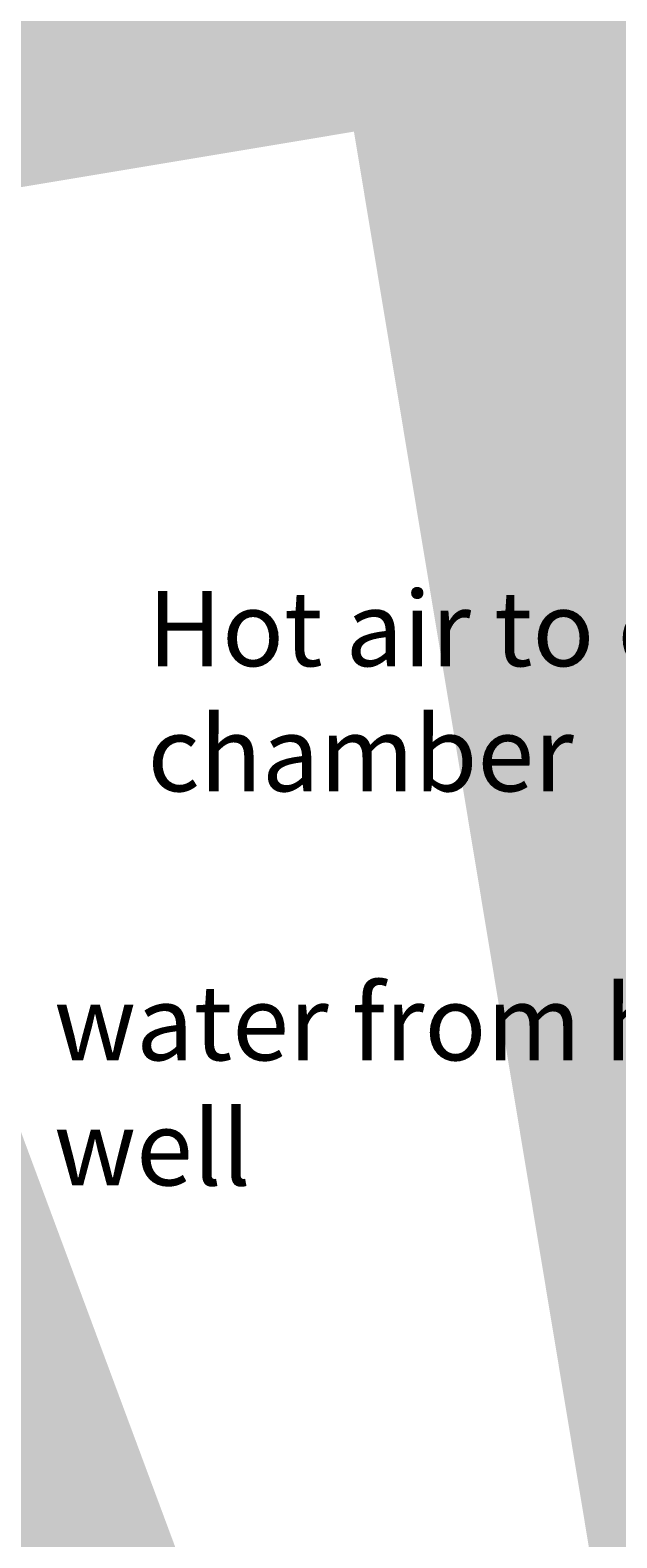
# Model space of a CAD drawing. Units: millimetres. Extents: x -22994 to 29398, y -19990 to 20176.
# Tile 22 of 135: x 5 to 37, y 99 to 180. Entities that reach past the tile are written whole.
import ezdxf

# ---------------------------------------------------------------- set-up
doc = ezdxf.new("R2010")
doc.units = ezdxf.units.MM
doc.header["$MEASUREMENT"] = 0
doc.layers.add('M-ANNO-TEXT', color=7, linetype='Continuous', lineweight=25)
doc.layers.add('M-DIMS', color=2, linetype='Continuous', lineweight=18)
doc.styles.get("Standard").update_dxf_attribs({"font": 'arial.ttf'})
doc.dimstyles.get("Standard").update_dxf_attribs({"dimtxt": 0.18, "dimasz": 10000, "dimexe": 0.18, "dimexo": 0.0625, "dimgap": 0.09, "dimtad": 0, "dimtih": 1, "dimtoh": 1, "dimdec": 0, "dimzin": 0, "dimdsep": 46, "dimtxsty": 'Standard', "dimcen": 0.09, "dimadec": 0, "dimazin": 0, "dimtfac": 1, "dimtdec": 0, "dimtofl": 0, "dimtmove": 0, "dimatfit": 3, "dimfxl": 1, "dimtolj": 1, "dimtzin": 0, "dimlwd": 30, "dimarcsym": 0})

# ---------------------------------------------------------------- blocks, each defined once
blk = doc.blocks.new('*D2')
at = {"layer": 'Defpoints', "color": 0, "transparency": 16777216}
for p in [(6.677, 10.271), (290.852, 10.271), (290.852, -5.079)]:
    blk.add_point(p, dxfattribs=at)
at = {"layer": 'M-DIMS', "color": 0, "lineweight": -2, "transparency": 16777216}
for p, q in [((6.677, 10.209), (6.677, -5.259)), ((290.852, 10.209), (290.852, -5.259))]:
    blk.add_line(p, q, dxfattribs=at)
at = {"layer": 'M-DIMS', "color": 0, "lineweight": 30, "transparency": 16777216}
for p, q in [((-9993.323, -5.079), (-19993.323, -5.079)), ((10290.852, -5.079), (20290.852, -5.079))]:
    blk.add_line(p, q, dxfattribs=at)
at = {"layer": 'M-DIMS', "color": 0, "transparency": 16777216}
for points in [[(-9993.323, 1661.588), (-9993.323, -1671.745), (6.677, -5.079)], [(10290.852, 1661.588), (10290.852, -1671.745), (290.852, -5.079)]]:
    blk.add_solid(points, dxfattribs=at)
at = {"layer": 'M-DIMS', "color": 0, "transparency": 16777216, "insert": (148.765, -5.079), "char_height": 0.18, "attachment_point": 5}
blk.add_mtext('\\A1;284.2', dxfattribs=at)
blk = doc.blocks.new('*D3')
at = {"layer": 'Defpoints', "color": 0, "transparency": 16777216}
for p in [(110.265, 204.165), (110.265, 176.366), (95.833, 127.967)]:
    blk.add_point(p, dxfattribs=at)
at = {"layer": 'M-DIMS', "color": 0, "lineweight": 30, "transparency": 16777216}
for p, q in [((-9904.167, 204.165), (-19904.167, 204.165)), ((10110.265, 204.165), (20110.265, 204.165))]:
    blk.add_line(p, q, dxfattribs=at)
at = {"layer": 'M-DIMS', "color": 0, "lineweight": -2, "transparency": 16777216}
for p, q in [((95.833, 128.03), (95.833, 204.345)), ((110.265, 176.429), (110.265, 204.345))]:
    blk.add_line(p, q, dxfattribs=at)
at = {"layer": 'M-DIMS', "color": 0, "transparency": 16777216}
for points in [[(-9904.167, 1870.832), (-9904.167, -1462.501), (95.833, 204.165)], [(10110.265, 1870.832), (10110.265, -1462.501), (110.265, 204.165)]]:
    blk.add_solid(points, dxfattribs=at)
at = {"layer": 'M-DIMS', "color": 0, "transparency": 16777216, "insert": (103.049, 204.165), "char_height": 0.18, "attachment_point": 5}
blk.add_mtext('\\A1;14.432', dxfattribs=at)
blk = doc.blocks.new('*D4')
at = {"layer": 'Defpoints', "color": 0, "transparency": 16777216}
for p in [(116.265, 204.165), (110.265, 176.366), (116.265, 176.366)]:
    blk.add_point(p, dxfattribs=at)
at = {"layer": 'M-DIMS', "color": 0, "lineweight": 30, "transparency": 16777216}
for p, q in [((-9889.735, 204.165), (-19889.735, 204.165)), ((10116.265, 204.165), (20116.265, 204.165))]:
    blk.add_line(p, q, dxfattribs=at)
at = {"layer": 'M-DIMS', "color": 0, "lineweight": -2, "transparency": 16777216}
for p, q in [((110.265, 176.429), (110.265, 204.345)), ((116.265, 176.429), (116.265, 204.345))]:
    blk.add_line(p, q, dxfattribs=at)
at = {"layer": 'M-DIMS', "color": 0, "transparency": 16777216}
for points in [[(-9889.735, 1870.832), (-9889.735, -1462.501), (110.265, 204.165)], [(10116.265, 1870.832), (10116.265, -1462.501), (116.265, 204.165)]]:
    blk.add_solid(points, dxfattribs=at)
at = {"layer": 'M-DIMS', "color": 0, "transparency": 16777216, "insert": (113.265, 204.165), "char_height": 0.18, "attachment_point": 5}
blk.add_mtext('\\A1;6', dxfattribs=at)
blk = doc.blocks.new('*D5')
at = {"layer": 'Defpoints', "color": 0, "transparency": 16777216}
for p in [(181.265, 204.165), (116.265, 176.366), (181.265, 176.366)]:
    blk.add_point(p, dxfattribs=at)
at = {"layer": 'M-DIMS', "color": 0, "lineweight": 30, "transparency": 16777216}
for p, q in [((-9883.735, 204.165), (-19883.735, 204.165)), ((10181.265, 204.165), (20181.265, 204.165))]:
    blk.add_line(p, q, dxfattribs=at)
at = {"layer": 'M-DIMS', "color": 0, "lineweight": -2, "transparency": 16777216}
for p, q in [((116.265, 176.429), (116.265, 204.345)), ((181.265, 176.429), (181.265, 204.345))]:
    blk.add_line(p, q, dxfattribs=at)
at = {"layer": 'M-DIMS', "color": 0, "transparency": 16777216}
for points in [[(-9883.735, 1870.832), (-9883.735, -1462.501), (116.265, 204.165)], [(10181.265, 1870.832), (10181.265, -1462.501), (181.265, 204.165)]]:
    blk.add_solid(points, dxfattribs=at)
at = {"layer": 'M-DIMS', "color": 0, "transparency": 16777216, "insert": (148.765, 204.165), "char_height": 0.18, "attachment_point": 5}
blk.add_mtext('\\A1;65', dxfattribs=at)
blk = doc.blocks.new('*D6')
at = {"layer": 'Defpoints', "color": 0, "transparency": 16777216}
for p in [(187.265, 204.165), (181.265, 176.366), (187.265, 176.366)]:
    blk.add_point(p, dxfattribs=at)
at = {"layer": 'M-DIMS', "color": 0, "lineweight": 30, "transparency": 16777216}
for p, q in [((-9818.735, 204.165), (-19818.735, 204.165)), ((10187.265, 204.165), (20187.265, 204.165))]:
    blk.add_line(p, q, dxfattribs=at)
at = {"layer": 'M-DIMS', "color": 0, "lineweight": -2, "transparency": 16777216}
for p, q in [((181.265, 176.429), (181.265, 204.345)), ((187.265, 176.429), (187.265, 204.345))]:
    blk.add_line(p, q, dxfattribs=at)
at = {"layer": 'M-DIMS', "color": 0, "transparency": 16777216}
for points in [[(-9818.735, 1870.832), (-9818.735, -1462.501), (181.265, 204.165)], [(10187.265, 1870.832), (10187.265, -1462.501), (187.265, 204.165)]]:
    blk.add_solid(points, dxfattribs=at)
at = {"layer": 'M-DIMS', "color": 0, "transparency": 16777216, "insert": (184.265, 204.165), "char_height": 0.18, "attachment_point": 5}
blk.add_mtext('\\A1;6', dxfattribs=at)
blk = doc.blocks.new('*D7')
at = {"layer": 'Defpoints', "color": 0, "transparency": 16777216}
for p in [(201.697, 204.165), (187.265, 176.366), (201.697, 127.967)]:
    blk.add_point(p, dxfattribs=at)
at = {"layer": 'M-DIMS', "color": 0, "lineweight": 30, "transparency": 16777216}
for p, q in [((-9812.735, 204.165), (-19812.735, 204.165)), ((10201.697, 204.165), (20201.697, 204.165))]:
    blk.add_line(p, q, dxfattribs=at)
at = {"layer": 'M-DIMS', "color": 0, "lineweight": -2, "transparency": 16777216}
for p, q in [((187.265, 176.429), (187.265, 204.345)), ((201.697, 128.03), (201.697, 204.345))]:
    blk.add_line(p, q, dxfattribs=at)
at = {"layer": 'M-DIMS', "color": 0, "transparency": 16777216}
for points in [[(-9812.735, 1870.832), (-9812.735, -1462.501), (187.265, 204.165)], [(10201.697, 1870.832), (10201.697, -1462.501), (201.697, 204.165)]]:
    blk.add_solid(points, dxfattribs=at)
at = {"layer": 'M-DIMS', "color": 0, "transparency": 16777216, "insert": (194.481, 204.165), "char_height": 0.18, "attachment_point": 5}
blk.add_mtext('\\A1;14.432', dxfattribs=at)
blk = doc.blocks.new('*D8')
at = {"layer": 'Defpoints', "color": 0, "transparency": 16777216}
for p in [(227.648, 204.165), (227.648, 146.73), (201.697, 127.967)]:
    blk.add_point(p, dxfattribs=at)
at = {"layer": 'M-DIMS', "color": 0, "lineweight": 30, "transparency": 16777216}
for p, q in [((-9798.303, 204.165), (-19798.303, 204.165)), ((10227.648, 204.165), (20227.648, 204.165))]:
    blk.add_line(p, q, dxfattribs=at)
at = {"layer": 'M-DIMS', "color": 0, "lineweight": -2, "transparency": 16777216}
for p, q in [((201.697, 128.03), (201.697, 204.345)), ((227.648, 146.792), (227.648, 204.345))]:
    blk.add_line(p, q, dxfattribs=at)
at = {"layer": 'M-DIMS', "color": 0, "transparency": 16777216}
for points in [[(-9798.303, 1870.832), (-9798.303, -1462.501), (201.697, 204.165)], [(10227.648, 1870.832), (10227.648, -1462.501), (227.648, 204.165)]]:
    blk.add_solid(points, dxfattribs=at)
at = {"layer": 'M-DIMS', "color": 0, "transparency": 16777216, "insert": (214.673, 204.165), "char_height": 0.18, "attachment_point": 5}
blk.add_mtext('\\A1;25.95', dxfattribs=at)
blk = doc.blocks.new('*D9')
at = {"layer": 'Defpoints', "color": 0, "transparency": 16777216}
for p in [(187.265, 176.366), (306.202, 176.366), (290.852, 10.271)]:
    blk.add_point(p, dxfattribs=at)
at = {"layer": 'M-DIMS', "color": 0, "lineweight": 30, "transparency": 16777216}
for p, q in [((306.202, 10176.366), (306.202, 20176.366)), ((306.202, -9989.729), (306.202, -19989.729))]:
    blk.add_line(p, q, dxfattribs=at)
at = {"layer": 'M-DIMS', "color": 0, "lineweight": -2, "transparency": 16777216}
for p, q in [((187.327, 176.366), (306.382, 176.366)), ((290.915, 10.271), (306.382, 10.271))]:
    blk.add_line(p, q, dxfattribs=at)
at = {"layer": 'M-DIMS', "color": 0, "transparency": 16777216}
for points in [[(-1360.465, 10176.366), (1972.869, 10176.366), (306.202, 176.366)], [(-1360.465, -9989.729), (1972.869, -9989.729), (306.202, 10.271)]]:
    blk.add_solid(points, dxfattribs=at)
at = {"layer": 'M-DIMS', "color": 0, "transparency": 16777216, "insert": (306.202, 93.319), "char_height": 0.18, "attachment_point": 5}
blk.add_mtext('\\A1;166.1', dxfattribs=at)
blk = doc.blocks.new('*D10')
at = {"layer": 'Defpoints', "color": 0, "transparency": 16777216}
for p in [(125.65, 136.071), (133.346, 136.071), (133.346, -5.079)]:
    blk.add_point(p, dxfattribs=at)
at = {"layer": 'M-DIMS', "color": 0, "lineweight": -2, "transparency": 16777216}
for p, q in [((125.65, 136.009), (125.65, -5.259)), ((133.346, 136.009), (133.346, -5.259))]:
    blk.add_line(p, q, dxfattribs=at)
at = {"layer": 'M-DIMS', "color": 0, "lineweight": 30, "transparency": 16777216}
for p, q in [((-9874.35, -5.079), (-19874.35, -5.079)), ((10133.346, -5.079), (20133.346, -5.079))]:
    blk.add_line(p, q, dxfattribs=at)
at = {"layer": 'M-DIMS', "color": 0, "transparency": 16777216}
for points in [[(-9874.35, 1661.588), (-9874.35, -1671.745), (125.65, -5.079)], [(10133.346, 1661.588), (10133.346, -1671.745), (133.346, -5.079)]]:
    blk.add_solid(points, dxfattribs=at)
at = {"layer": 'M-DIMS', "color": 0, "transparency": 16777216, "insert": (129.498, -5.079), "char_height": 0.18, "attachment_point": 5}
blk.add_mtext('\\A1;7.696', dxfattribs=at)
blk = doc.blocks.new('*D11')
at = {"layer": 'Defpoints', "color": 0, "transparency": 16777216}
for p in [(133.346, 136.071), (135.65, 136.071), (135.65, -5.079)]:
    blk.add_point(p, dxfattribs=at)
at = {"layer": 'M-DIMS', "color": 0, "lineweight": -2, "transparency": 16777216}
for p, q in [((133.346, 136.009), (133.346, -5.259)), ((135.65, 136.009), (135.65, -5.259))]:
    blk.add_line(p, q, dxfattribs=at)
at = {"layer": 'M-DIMS', "color": 0, "lineweight": 30, "transparency": 16777216}
for p, q in [((-9866.654, -5.079), (-19866.654, -5.079)), ((10135.65, -5.079), (20135.65, -5.079))]:
    blk.add_line(p, q, dxfattribs=at)
at = {"layer": 'M-DIMS', "color": 0, "transparency": 16777216}
for points in [[(-9866.654, 1661.588), (-9866.654, -1671.745), (133.346, -5.079)], [(10135.65, 1661.588), (10135.65, -1671.745), (135.65, -5.079)]]:
    blk.add_solid(points, dxfattribs=at)
at = {"layer": 'M-DIMS', "color": 0, "transparency": 16777216, "insert": (134.498, -5.079), "char_height": 0.18, "attachment_point": 5}
blk.add_mtext('\\A1;2.304', dxfattribs=at)
blk = doc.blocks.new('*D12')
at = {"layer": 'Defpoints', "color": 0, "transparency": 16777216}
for p in [(135.65, 136.071), (145.65, 136.071), (145.65, -5.079)]:
    blk.add_point(p, dxfattribs=at)
at = {"layer": 'M-DIMS', "color": 0, "lineweight": -2, "transparency": 16777216}
for p, q in [((135.65, 136.009), (135.65, -5.259)), ((145.65, 136.009), (145.65, -5.259))]:
    blk.add_line(p, q, dxfattribs=at)
at = {"layer": 'M-DIMS', "color": 0, "lineweight": 30, "transparency": 16777216}
for p, q in [((-9864.35, -5.079), (-19864.35, -5.079)), ((10145.65, -5.079), (20145.65, -5.079))]:
    blk.add_line(p, q, dxfattribs=at)
at = {"layer": 'M-DIMS', "color": 0, "transparency": 16777216}
for points in [[(-9864.35, 1661.588), (-9864.35, -1671.745), (135.65, -5.079)], [(10145.65, 1661.588), (10145.65, -1671.745), (145.65, -5.079)]]:
    blk.add_solid(points, dxfattribs=at)
at = {"layer": 'M-DIMS', "color": 0, "transparency": 16777216, "insert": (140.65, -5.079), "char_height": 0.18, "attachment_point": 5}
blk.add_mtext('\\A1;10', dxfattribs=at)
blk = doc.blocks.new('*D13')
at = {"layer": 'Defpoints', "color": 0, "transparency": 16777216}
for p in [(145.65, 136.071), (155.65, 136.071), (155.65, -5.079)]:
    blk.add_point(p, dxfattribs=at)
at = {"layer": 'M-DIMS', "color": 0, "lineweight": -2, "transparency": 16777216}
for p, q in [((145.65, 136.009), (145.65, -5.259)), ((155.65, 136.009), (155.65, -5.259))]:
    blk.add_line(p, q, dxfattribs=at)
at = {"layer": 'M-DIMS', "color": 0, "lineweight": 30, "transparency": 16777216}
for p, q in [((-9854.35, -5.079), (-19854.35, -5.079)), ((10155.65, -5.079), (20155.65, -5.079))]:
    blk.add_line(p, q, dxfattribs=at)
at = {"layer": 'M-DIMS', "color": 0, "transparency": 16777216}
for points in [[(-9854.35, 1661.588), (-9854.35, -1671.745), (145.65, -5.079)], [(10155.65, 1661.588), (10155.65, -1671.745), (155.65, -5.079)]]:
    blk.add_solid(points, dxfattribs=at)
at = {"layer": 'M-DIMS', "color": 0, "transparency": 16777216, "insert": (150.65, -5.079), "char_height": 0.18, "attachment_point": 5}
blk.add_mtext('\\A1;10', dxfattribs=at)
blk = doc.blocks.new('*D14')
at = {"layer": 'Defpoints', "color": 0, "transparency": 16777216}
for p in [(155.65, 136.071), (165.65, 136.071), (165.65, -5.079)]:
    blk.add_point(p, dxfattribs=at)
at = {"layer": 'M-DIMS', "color": 0, "lineweight": -2, "transparency": 16777216}
for p, q in [((155.65, 136.009), (155.65, -5.259)), ((165.65, 136.009), (165.65, -5.259))]:
    blk.add_line(p, q, dxfattribs=at)
at = {"layer": 'M-DIMS', "color": 0, "lineweight": 30, "transparency": 16777216}
for p, q in [((-9844.35, -5.079), (-19844.35, -5.079)), ((10165.65, -5.079), (20165.65, -5.079))]:
    blk.add_line(p, q, dxfattribs=at)
at = {"layer": 'M-DIMS', "color": 0, "transparency": 16777216}
for points in [[(-9844.35, 1661.588), (-9844.35, -1671.745), (155.65, -5.079)], [(10165.65, 1661.588), (10165.65, -1671.745), (165.65, -5.079)]]:
    blk.add_solid(points, dxfattribs=at)
at = {"layer": 'M-DIMS', "color": 0, "transparency": 16777216, "insert": (160.65, -5.079), "char_height": 0.18, "attachment_point": 5}
blk.add_mtext('\\A1;10', dxfattribs=at)
blk = doc.blocks.new('*D15')
at = {"layer": 'Defpoints', "color": 0, "transparency": 16777216}
for p in [(173.346, 154.788), (173.346, 136.071), (306.202, 136.071)]:
    blk.add_point(p, dxfattribs=at)
at = {"layer": 'M-DIMS', "color": 0, "lineweight": 30, "transparency": 16777216}
for p, q in [((306.202, 10154.788), (306.202, 20154.788)), ((306.202, -9863.929), (306.202, -19863.929))]:
    blk.add_line(p, q, dxfattribs=at)
at = {"layer": 'M-DIMS', "color": 0, "lineweight": -2, "transparency": 16777216}
for p, q in [((173.408, 154.788), (306.382, 154.788)), ((173.408, 136.071), (306.382, 136.071))]:
    blk.add_line(p, q, dxfattribs=at)
at = {"layer": 'M-DIMS', "color": 0, "transparency": 16777216}
for points in [[(-1360.465, 10154.788), (1972.869, 10154.788), (306.202, 154.788)], [(-1360.465, -9863.929), (1972.869, -9863.929), (306.202, 136.071)]]:
    blk.add_solid(points, dxfattribs=at)
at = {"layer": 'M-DIMS', "color": 0, "transparency": 16777216, "insert": (306.202, 145.43), "char_height": 0.18, "attachment_point": 5}
blk.add_mtext('\\A1;18.717', dxfattribs=at)
blk = doc.blocks.new('*D16')
at = {"layer": 'Defpoints', "color": 0, "transparency": 16777216}
for p in [(120.17, 204.165), (110.466, 48.035), (120.17, 48.035)]:
    blk.add_point(p, dxfattribs=at)
at = {"layer": 'M-DIMS', "color": 0, "lineweight": 30, "transparency": 16777216}
for p, q in [((-9889.534, 204.165), (-19889.534, 204.165)), ((10120.17, 204.165), (20120.17, 204.165))]:
    blk.add_line(p, q, dxfattribs=at)
at = {"layer": 'M-DIMS', "color": 0, "lineweight": -2, "transparency": 16777216}
for p, q in [((110.466, 48.097), (110.466, 204.345)), ((120.17, 48.097), (120.17, 204.345))]:
    blk.add_line(p, q, dxfattribs=at)
at = {"layer": 'M-DIMS', "color": 0, "transparency": 16777216}
for points in [[(-9889.534, 1870.832), (-9889.534, -1462.501), (110.466, 204.165)], [(10120.17, 1870.832), (10120.17, -1462.501), (120.17, 204.165)]]:
    blk.add_solid(points, dxfattribs=at)
at = {"layer": 'M-DIMS', "color": 0, "transparency": 16777216, "insert": (115.318, 204.165), "char_height": 0.18, "attachment_point": 5}
blk.add_mtext('\\A1;9.704', dxfattribs=at)
blk = doc.blocks.new('*D17')
at = {"layer": 'Defpoints', "color": 0, "transparency": 16777216}
for p in [(126.17, 204.165), (120.17, 48.035), (126.17, 48.035)]:
    blk.add_point(p, dxfattribs=at)
at = {"layer": 'M-DIMS', "color": 0, "lineweight": 30, "transparency": 16777216}
for p, q in [((-9879.83, 204.165), (-19879.83, 204.165)), ((10126.17, 204.165), (20126.17, 204.165))]:
    blk.add_line(p, q, dxfattribs=at)
at = {"layer": 'M-DIMS', "color": 0, "lineweight": -2, "transparency": 16777216}
for p, q in [((120.17, 48.097), (120.17, 204.345)), ((126.17, 48.097), (126.17, 204.345))]:
    blk.add_line(p, q, dxfattribs=at)
at = {"layer": 'M-DIMS', "color": 0, "transparency": 16777216}
for points in [[(-9879.83, 1870.832), (-9879.83, -1462.501), (120.17, 204.165)], [(10126.17, 1870.832), (10126.17, -1462.501), (126.17, 204.165)]]:
    blk.add_solid(points, dxfattribs=at)
at = {"layer": 'M-DIMS', "color": 0, "transparency": 16777216, "insert": (123.17, 204.165), "char_height": 0.18, "attachment_point": 5}
blk.add_mtext('\\A1;6', dxfattribs=at)
blk = doc.blocks.new('*D18')
at = {"layer": 'Defpoints', "color": 0, "transparency": 16777216}
for p in [(132.17, 204.165), (126.17, 48.035), (132.17, 48.035)]:
    blk.add_point(p, dxfattribs=at)
at = {"layer": 'M-DIMS', "color": 0, "lineweight": 30, "transparency": 16777216}
for p, q in [((-9873.83, 204.165), (-19873.83, 204.165)), ((10132.17, 204.165), (20132.17, 204.165))]:
    blk.add_line(p, q, dxfattribs=at)
at = {"layer": 'M-DIMS', "color": 0, "lineweight": -2, "transparency": 16777216}
for p, q in [((126.17, 48.097), (126.17, 204.345)), ((132.17, 48.097), (132.17, 204.345))]:
    blk.add_line(p, q, dxfattribs=at)
at = {"layer": 'M-DIMS', "color": 0, "transparency": 16777216}
for points in [[(-9873.83, 1870.832), (-9873.83, -1462.501), (126.17, 204.165)], [(10132.17, 1870.832), (10132.17, -1462.501), (132.17, 204.165)]]:
    blk.add_solid(points, dxfattribs=at)
at = {"layer": 'M-DIMS', "color": 0, "transparency": 16777216, "insert": (129.17, 204.165), "char_height": 0.18, "attachment_point": 5}
blk.add_mtext('\\A1;6', dxfattribs=at)
blk = doc.blocks.new('*D19')
at = {"layer": 'Defpoints', "color": 0, "transparency": 16777216}
for p in [(138.17, 204.165), (132.17, 48.035), (138.17, 48.035)]:
    blk.add_point(p, dxfattribs=at)
at = {"layer": 'M-DIMS', "color": 0, "lineweight": 30, "transparency": 16777216}
for p, q in [((-9867.83, 204.165), (-19867.83, 204.165)), ((10138.17, 204.165), (20138.17, 204.165))]:
    blk.add_line(p, q, dxfattribs=at)
at = {"layer": 'M-DIMS', "color": 0, "lineweight": -2, "transparency": 16777216}
for p, q in [((132.17, 48.097), (132.17, 204.345)), ((138.17, 48.097), (138.17, 204.345))]:
    blk.add_line(p, q, dxfattribs=at)
at = {"layer": 'M-DIMS', "color": 0, "transparency": 16777216}
for points in [[(-9867.83, 1870.832), (-9867.83, -1462.501), (132.17, 204.165)], [(10138.17, 1870.832), (10138.17, -1462.501), (138.17, 204.165)]]:
    blk.add_solid(points, dxfattribs=at)
at = {"layer": 'M-DIMS', "color": 0, "transparency": 16777216, "insert": (135.17, 204.165), "char_height": 0.18, "attachment_point": 5}
blk.add_mtext('\\A1;6', dxfattribs=at)
blk = doc.blocks.new('*D20')
at = {"layer": 'Defpoints', "color": 0, "transparency": 16777216}
for p in [(144.17, 204.165), (138.17, 48.035), (144.17, 48.035)]:
    blk.add_point(p, dxfattribs=at)
at = {"layer": 'M-DIMS', "color": 0, "lineweight": 30, "transparency": 16777216}
for p, q in [((-9861.83, 204.165), (-19861.83, 204.165)), ((10144.17, 204.165), (20144.17, 204.165))]:
    blk.add_line(p, q, dxfattribs=at)
at = {"layer": 'M-DIMS', "color": 0, "lineweight": -2, "transparency": 16777216}
for p, q in [((138.17, 48.097), (138.17, 204.345)), ((144.17, 48.097), (144.17, 204.345))]:
    blk.add_line(p, q, dxfattribs=at)
at = {"layer": 'M-DIMS', "color": 0, "transparency": 16777216}
for points in [[(-9861.83, 1870.832), (-9861.83, -1462.501), (138.17, 204.165)], [(10144.17, 1870.832), (10144.17, -1462.501), (144.17, 204.165)]]:
    blk.add_solid(points, dxfattribs=at)
at = {"layer": 'M-DIMS', "color": 0, "transparency": 16777216, "insert": (141.17, 204.165), "char_height": 0.18, "attachment_point": 5}
blk.add_mtext('\\A1;6', dxfattribs=at)
blk = doc.blocks.new('*D21')
at = {"layer": 'Defpoints', "color": 0, "transparency": 16777216}
for p in [(149.116, 204.165), (144.17, 48.035), (149.116, 48.035)]:
    blk.add_point(p, dxfattribs=at)
at = {"layer": 'M-DIMS', "color": 0, "lineweight": 30, "transparency": 16777216}
for p, q in [((-9855.83, 204.165), (-19855.83, 204.165)), ((10149.116, 204.165), (20149.116, 204.165))]:
    blk.add_line(p, q, dxfattribs=at)
at = {"layer": 'M-DIMS', "color": 0, "lineweight": -2, "transparency": 16777216}
for p, q in [((144.17, 48.097), (144.17, 204.345)), ((149.116, 48.097), (149.116, 204.345))]:
    blk.add_line(p, q, dxfattribs=at)
at = {"layer": 'M-DIMS', "color": 0, "transparency": 16777216}
for points in [[(-9855.83, 1870.832), (-9855.83, -1462.501), (144.17, 204.165)], [(10149.116, 1870.832), (10149.116, -1462.501), (149.116, 204.165)]]:
    blk.add_solid(points, dxfattribs=at)
at = {"layer": 'M-DIMS', "color": 0, "transparency": 16777216, "insert": (146.643, 204.165), "char_height": 0.18, "attachment_point": 5}
blk.add_mtext('\\A1;4.945', dxfattribs=at)
blk = doc.blocks.new('*D22')
at = {"layer": 'Defpoints', "color": 0, "transparency": 16777216}
for p in [(149.116, 30.99), (155.116, 30.99), (155.116, -5.079)]:
    blk.add_point(p, dxfattribs=at)
at = {"layer": 'M-DIMS', "color": 0, "lineweight": -2, "transparency": 16777216}
for p, q in [((149.116, 30.927), (149.116, -5.259)), ((155.116, 30.927), (155.116, -5.259))]:
    blk.add_line(p, q, dxfattribs=at)
at = {"layer": 'M-DIMS', "color": 0, "lineweight": 30, "transparency": 16777216}
for p, q in [((-9850.884, -5.079), (-19850.884, -5.079)), ((10155.116, -5.079), (20155.116, -5.079))]:
    blk.add_line(p, q, dxfattribs=at)
at = {"layer": 'M-DIMS', "color": 0, "transparency": 16777216}
for points in [[(-9850.884, 1661.588), (-9850.884, -1671.745), (149.116, -5.079)], [(10155.116, 1661.588), (10155.116, -1671.745), (155.116, -5.079)]]:
    blk.add_solid(points, dxfattribs=at)
at = {"layer": 'M-DIMS', "color": 0, "transparency": 16777216, "insert": (152.116, -5.079), "char_height": 0.18, "attachment_point": 5}
blk.add_mtext('\\A1;6', dxfattribs=at)
blk = doc.blocks.new('*D23')
at = {"layer": 'Defpoints', "color": 0, "transparency": 16777216}
for p in [(155.116, 30.99), (161.116, 30.99), (161.116, -5.079)]:
    blk.add_point(p, dxfattribs=at)
at = {"layer": 'M-DIMS', "color": 0, "lineweight": -2, "transparency": 16777216}
for p, q in [((155.116, 30.927), (155.116, -5.259)), ((161.116, 30.927), (161.116, -5.259))]:
    blk.add_line(p, q, dxfattribs=at)
at = {"layer": 'M-DIMS', "color": 0, "lineweight": 30, "transparency": 16777216}
for p, q in [((-9844.884, -5.079), (-19844.884, -5.079)), ((10161.116, -5.079), (20161.116, -5.079))]:
    blk.add_line(p, q, dxfattribs=at)
at = {"layer": 'M-DIMS', "color": 0, "transparency": 16777216}
for points in [[(-9844.884, 1661.588), (-9844.884, -1671.745), (155.116, -5.079)], [(10161.116, 1661.588), (10161.116, -1671.745), (161.116, -5.079)]]:
    blk.add_solid(points, dxfattribs=at)
at = {"layer": 'M-DIMS', "color": 0, "transparency": 16777216, "insert": (158.116, -5.079), "char_height": 0.18, "attachment_point": 5}
blk.add_mtext('\\A1;6', dxfattribs=at)
blk = doc.blocks.new('*D24')
at = {"layer": 'Defpoints', "color": 0, "transparency": 16777216}
for p in [(161.116, 30.99), (166.439, 30.99), (166.439, -5.079)]:
    blk.add_point(p, dxfattribs=at)
at = {"layer": 'M-DIMS', "color": 0, "lineweight": -2, "transparency": 16777216}
for p, q in [((161.116, 30.927), (161.116, -5.259)), ((166.439, 30.927), (166.439, -5.259))]:
    blk.add_line(p, q, dxfattribs=at)
at = {"layer": 'M-DIMS', "color": 0, "lineweight": 30, "transparency": 16777216}
for p, q in [((-9838.884, -5.079), (-19838.884, -5.079)), ((10166.439, -5.079), (20166.439, -5.079))]:
    blk.add_line(p, q, dxfattribs=at)
at = {"layer": 'M-DIMS', "color": 0, "transparency": 16777216}
for points in [[(-9838.884, 1661.588), (-9838.884, -1671.745), (161.116, -5.079)], [(10166.439, 1661.588), (10166.439, -1671.745), (166.439, -5.079)]]:
    blk.add_solid(points, dxfattribs=at)
at = {"layer": 'M-DIMS', "color": 0, "transparency": 16777216, "insert": (163.777, -5.079), "char_height": 0.18, "attachment_point": 5}
blk.add_mtext('\\A1;5.323', dxfattribs=at)
blk = doc.blocks.new('*D25')
at = {"layer": 'Defpoints', "color": 0, "transparency": 16777216}
for p in [(166.439, 30.99), (172.439, 30.99), (172.439, -5.079)]:
    blk.add_point(p, dxfattribs=at)
at = {"layer": 'M-DIMS', "color": 0, "lineweight": -2, "transparency": 16777216}
for p, q in [((166.439, 30.927), (166.439, -5.259)), ((172.439, 30.927), (172.439, -5.259))]:
    blk.add_line(p, q, dxfattribs=at)
at = {"layer": 'M-DIMS', "color": 0, "lineweight": 30, "transparency": 16777216}
for p, q in [((-9833.561, -5.079), (-19833.561, -5.079)), ((10172.439, -5.079), (20172.439, -5.079))]:
    blk.add_line(p, q, dxfattribs=at)
at = {"layer": 'M-DIMS', "color": 0, "transparency": 16777216}
for points in [[(-9833.561, 1661.588), (-9833.561, -1671.745), (166.439, -5.079)], [(10172.439, 1661.588), (10172.439, -1671.745), (172.439, -5.079)]]:
    blk.add_solid(points, dxfattribs=at)
at = {"layer": 'M-DIMS', "color": 0, "transparency": 16777216, "insert": (169.439, -5.079), "char_height": 0.18, "attachment_point": 5}
blk.add_mtext('\\A1;6', dxfattribs=at)
blk = doc.blocks.new('*D26')
at = {"layer": 'Defpoints', "color": 0, "transparency": 16777216}
for p in [(172.439, 30.99), (178.439, 30.99), (178.439, -5.079)]:
    blk.add_point(p, dxfattribs=at)
at = {"layer": 'M-DIMS', "color": 0, "lineweight": -2, "transparency": 16777216}
for p, q in [((172.439, 30.927), (172.439, -5.259)), ((178.439, 30.927), (178.439, -5.259))]:
    blk.add_line(p, q, dxfattribs=at)
at = {"layer": 'M-DIMS', "color": 0, "lineweight": 30, "transparency": 16777216}
for p, q in [((-9827.561, -5.079), (-19827.561, -5.079)), ((10178.439, -5.079), (20178.439, -5.079))]:
    blk.add_line(p, q, dxfattribs=at)
at = {"layer": 'M-DIMS', "color": 0, "transparency": 16777216}
for points in [[(-9827.561, 1661.588), (-9827.561, -1671.745), (172.439, -5.079)], [(10178.439, 1661.588), (10178.439, -1671.745), (178.439, -5.079)]]:
    blk.add_solid(points, dxfattribs=at)
at = {"layer": 'M-DIMS', "color": 0, "transparency": 16777216, "insert": (175.439, -5.079), "char_height": 0.18, "attachment_point": 5}
blk.add_mtext('\\A1;6', dxfattribs=at)
blk = doc.blocks.new('*D27')
at = {"layer": 'Defpoints', "color": 0, "transparency": 16777216}
for p in [(178.439, 30.99), (188.117, 30.99), (188.117, -5.079)]:
    blk.add_point(p, dxfattribs=at)
at = {"layer": 'M-DIMS', "color": 0, "lineweight": -2, "transparency": 16777216}
for p, q in [((178.439, 30.927), (178.439, -5.259)), ((188.117, 30.927), (188.117, -5.259))]:
    blk.add_line(p, q, dxfattribs=at)
at = {"layer": 'M-DIMS', "color": 0, "lineweight": 30, "transparency": 16777216}
for p, q in [((-9821.561, -5.079), (-19821.561, -5.079)), ((10188.117, -5.079), (20188.117, -5.079))]:
    blk.add_line(p, q, dxfattribs=at)
at = {"layer": 'M-DIMS', "color": 0, "transparency": 16777216}
for points in [[(-9821.561, 1661.588), (-9821.561, -1671.745), (178.439, -5.079)], [(10188.117, 1661.588), (10188.117, -1671.745), (188.117, -5.079)]]:
    blk.add_solid(points, dxfattribs=at)
at = {"layer": 'M-DIMS', "color": 0, "transparency": 16777216, "insert": (183.278, -5.079), "char_height": 0.18, "attachment_point": 5}
blk.add_mtext('\\A1;9.679', dxfattribs=at)
blk = doc.blocks.new('*D28')
at = {"layer": 'Defpoints', "color": 0, "transparency": 16777216}
for p in [(188.117, 48.035), (306.202, 48.035), (188.117, 30.99)]:
    blk.add_point(p, dxfattribs=at)
at = {"layer": 'M-DIMS', "color": 0, "lineweight": 30, "transparency": 16777216}
for p, q in [((306.202, 10048.035), (306.202, 20048.035)), ((306.202, -9969.01), (306.202, -19969.01))]:
    blk.add_line(p, q, dxfattribs=at)
at = {"layer": 'M-DIMS', "color": 0, "lineweight": -2, "transparency": 16777216}
for p, q in [((188.18, 48.035), (306.382, 48.035)), ((188.18, 30.99), (306.382, 30.99))]:
    blk.add_line(p, q, dxfattribs=at)
at = {"layer": 'M-DIMS', "color": 0, "transparency": 16777216}
for points in [[(-1360.465, 10048.035), (1972.869, 10048.035), (306.202, 48.035)], [(-1360.465, -9969.01), (1972.869, -9969.01), (306.202, 30.99)]]:
    blk.add_solid(points, dxfattribs=at)
at = {"layer": 'M-DIMS', "color": 0, "transparency": 16777216, "insert": (306.202, 39.512), "char_height": 0.18, "attachment_point": 5}
blk.add_mtext('\\A1;17.045', dxfattribs=at)
blk = doc.blocks.new('*D32')
at = {"layer": 'Defpoints', "color": 0, "transparency": 16777216}
for p in [(57.164, 118.614), (52.413, 113.093)]:
    blk.add_point(p, dxfattribs=at)
at = {"layer": 'M-DIMS', "color": 0, "lineweight": -2, "transparency": 16777216}
for p, q in [((57.074, 118.614), (57.254, 118.614)), ((57.164, 118.524), (57.164, 118.704))]:
    blk.add_line(p, q, dxfattribs=at)
at = {"layer": 'M-DIMS', "color": 0, "lineweight": 30, "transparency": 16777216}
for p, q in [((-12992.534, -15047.031), (-6470.06, -7466.969)), ((-22992.534, -15047.031), (-12992.534, -15047.031))]:
    blk.add_line(p, q, dxfattribs=at)
at = {"layer": 'M-DIMS', "color": 0, "transparency": 16777216}
blk.add_solid([(-7733.404, -6379.89), (-5206.717, -8554.048), (52.413, 113.093)], dxfattribs=at)
at = {"layer": 'M-DIMS', "color": 0, "transparency": 16777216, "insert": (-22993.208, -15047.031), "char_height": 0.18, "attachment_point": 5}
blk.add_mtext('\\A1;2X R7.284', dxfattribs=at)
blk = doc.blocks.new('*D35')
at = {"layer": 'Defpoints', "color": 0, "transparency": 16777216}
for p in [(21.093, 77.393), (21.84, 76.092)]:
    blk.add_point(p, dxfattribs=at)
at = {"layer": 'M-DIMS', "color": 0, "lineweight": 30, "transparency": 16777216}
for p, q in [((-19938.013, 17421.447), (-9938.013, 17421.447)), ((-9938.013, 17421.447), (-4958.46, 8749.42))]:
    blk.add_line(p, q, dxfattribs=at)
at = {"layer": 'M-DIMS', "color": 0, "lineweight": -2, "transparency": 16777216}
for p, q in [((21.75, 76.092), (21.93, 76.092)), ((21.84, 76.002), (21.84, 76.182))]:
    blk.add_line(p, q, dxfattribs=at)
at = {"layer": 'M-DIMS', "color": 0, "transparency": 16777216}
blk.add_solid([(-3513.122, 9579.345), (-6403.798, 7919.494), (21.093, 77.393)], dxfattribs=at)
at = {"layer": 'M-DIMS', "color": 0, "transparency": 16777216, "insert": (-19938.354, 17421.447), "char_height": 0.18, "attachment_point": 5}
blk.add_mtext('\\A1;R1.5', dxfattribs=at)
blk = doc.blocks.new('*D36')
at = {"layer": 'Defpoints', "color": 0, "transparency": 16777216}
for p in [(46.39, 31.303), (46.387, 26.593)]:
    blk.add_point(p, dxfattribs=at)
at = {"layer": 'M-DIMS', "color": 0, "lineweight": 30, "transparency": 16777216}
for p, q in [((57.15, 20031.301), (51.77, 10031.302)), ((10057.15, 20031.301), (57.15, 20031.301))]:
    blk.add_line(p, q, dxfattribs=at)
at = {"layer": 'M-DIMS', "color": 0, "lineweight": -2, "transparency": 16777216}
for p, q in [((46.299, 28.948), (46.479, 28.948)), ((46.389, 28.858), (46.389, 29.038))]:
    blk.add_line(p, q, dxfattribs=at)
at = {"layer": 'M-DIMS', "color": 0, "transparency": 16777216}
blk.add_solid([(-1614.896, 10032.199), (1718.436, 10030.405), (46.39, 31.303)], dxfattribs=at)
at = {"layer": 'M-DIMS', "color": 0, "transparency": 16777216, "insert": (10057.554, 20031.301), "char_height": 0.18, "attachment_point": 5}
blk.add_mtext('\\A1;∅4.71', dxfattribs=at)

msp = doc.modelspace()

# ---------------------------------------------------------------- texts
at = {"layer": 'M-ANNO-TEXT', "char_height": 4, "attachment_point": 1}
for s, insert in [('Hot air to combustion chamber', (11.6233, 149.8324)), ('water from hot \\Pwell', (6.6341, 128.828))]:
    msp.add_mtext_dynamic_manual_height_columns(s, width=57.451589, gutter_width=1, heights=[0], dxfattribs=dict(at, insert=insert))

# ---------------------------------------------------------------- dimensions: what is measured, and where the dimension line sits
at = {"layer": 'M-DIMS'}
for base, p1, p2, override, picture, middle in [((306.202, 176.3662), (290.852, 10.2713), (187.2647, 176.3662), {"dimdec": 1, "dimlfac": 1, "dimrnd": 0, "dimzin": 0, "dimdsep": 46, "dimlunit": 2}, '*D9', (306.202, 93.3187)), ((306.202, 136.0713), (173.3459, 154.788), (173.3459, 136.0713), {"dimdec": 3, "dimlfac": 1, "dimrnd": 0, "dimzin": 0, "dimdsep": 46, "dimlunit": 2}, '*D15', (306.202, 145.4297)), ((306.202, 48.0349), (188.1175, 30.9895), (188.1175, 48.0349), {"dimdec": 3, "dimlfac": 1, "dimrnd": 0, "dimzin": 0, "dimdsep": 46, "dimlunit": 2}, '*D28', (306.202, 39.5122))]:
    dim = msp.add_linear_dim(base=base, p1=p1, p2=p2, angle=90, dimstyle='Standard', override=override, dxfattribs=at)
    dim.commit()
    dim.dimension.update_dxf_attribs({"geometry": picture, "text_midpoint": middle})
dim = msp.add_diameter_dim_2p(p1=(46.3875, 26.5934), p2=(46.39, 31.3035), dimstyle='Standard', override={"dimdec": 2, "dimlfac": 1, "dimrnd": 0, "dimzin": 0, "dimdsep": 46, "dimlunit": 2}, dxfattribs=at)
dim.commit()
dim.dimension.update_dxf_attribs({"geometry": '*D36', "text_midpoint": (10057.5542, 20031.3006), "dimtype": 163})
dim = msp.add_radius_dim(center=(21.8402, 76.0922), mpoint=(21.0933, 77.393), dimstyle='Standard', override={"dimdec": 1, "dimlfac": 1, "dimrnd": 0, "dimzin": 0, "dimdsep": 46, "dimlunit": 2}, dxfattribs=at)
dim.commit()
dim.dimension.update_dxf_attribs({"geometry": '*D35', "text_midpoint": (-19938.3541, 17421.4466)})
for base, p1, p2, override, picture, middle in [((110.2647, 204.1654), (95.8327, 127.967), (110.2647, 176.3662), {"dimdec": 3, "dimlfac": 1, "dimrnd": 0, "dimzin": 0, "dimdsep": 46, "dimlunit": 2}, '*D3', (103.0487, 204.1654)), ((116.2647, 204.1654), (110.2647, 176.3662), (116.2647, 176.3662), {"dimdec": 0, "dimlfac": 1, "dimrnd": 0, "dimzin": 0, "dimdsep": 46, "dimlunit": 2}, '*D4', (113.2647, 204.1654)), ((120.1702, 204.1654), (110.4658, 48.0349), (120.1702, 48.0349), {"dimdec": 3, "dimlfac": 1, "dimrnd": 0, "dimzin": 0, "dimdsep": 46, "dimlunit": 2}, '*D16', (115.318, 204.1654)), ((181.2647, 204.1654), (116.2647, 176.3662), (181.2647, 176.3662), {"dimdec": 0, "dimlfac": 1, "dimrnd": 0, "dimzin": 0, "dimdsep": 46, "dimlunit": 2}, '*D5', (148.7647, 204.1654)), ((126.1702, 204.1654), (120.1702, 48.0349), (126.1702, 48.0349), {"dimdec": 0, "dimlfac": 1, "dimrnd": 0, "dimzin": 0, "dimdsep": 46, "dimlunit": 2}, '*D17', (123.1702, 204.1654)), ((132.1702, 204.1654), (126.1702, 48.0349), (132.1702, 48.0349), {"dimdec": 0, "dimlfac": 1, "dimrnd": 0, "dimzin": 0, "dimdsep": 46, "dimlunit": 2}, '*D18', (129.1702, 204.1654)), ((138.1702, 204.1654), (132.1702, 48.0349), (138.1702, 48.0349), {"dimdec": 0, "dimlfac": 1, "dimrnd": 0, "dimzin": 0, "dimdsep": 46, "dimlunit": 2}, '*D19', (135.1702, 204.1654)), ((144.1702, 204.1654), (138.1702, 48.0349), (144.1702, 48.0349), {"dimdec": 0, "dimlfac": 1, "dimrnd": 0, "dimzin": 0, "dimdsep": 46, "dimlunit": 2}, '*D20', (141.1702, 204.1654)), ((149.11567, 204.16539), (144.17023, 48.03494), (149.11567, 48.03494), {"dimdec": 3, "dimlfac": 1, "dimrnd": 0, "dimzin": 0, "dimdsep": 46, "dimlunit": 2}, '*D21', (146.64295, 204.16539)), ((187.2647, 204.1654), (181.2647, 176.3662), (187.2647, 176.3662), {"dimdec": 0, "dimlfac": 1, "dimrnd": 0, "dimzin": 0, "dimdsep": 46, "dimlunit": 2}, '*D6', (184.2647, 204.1654)), ((201.6967, 204.1654), (187.2647, 176.3662), (201.6967, 127.967), {"dimdec": 3, "dimlfac": 1, "dimrnd": 0, "dimzin": 0, "dimdsep": 46, "dimlunit": 2}, '*D7', (194.4807, 204.1654)), ((227.6485, 204.1654), (201.6967, 127.967), (227.6485, 146.7296), {"dimdec": 2, "dimlfac": 1, "dimrnd": 0, "dimzin": 0, "dimdsep": 46, "dimlunit": 2}, '*D8', (214.6726, 204.1654)), ((290.852, -5.0787), (6.6773, 10.2713), (290.852, 10.2713), {"dimdec": 1, "dimlfac": 1, "dimrnd": 0, "dimzin": 0, "dimdsep": 46, "dimlunit": 2}, '*D2', (148.7647, -5.0787)), ((133.3459, -5.0787), (125.6498, 136.0713), (133.3459, 136.0713), {"dimdec": 3, "dimlfac": 1, "dimrnd": 0, "dimzin": 0, "dimdsep": 46, "dimlunit": 2}, '*D10', (129.4978, -5.0787)), ((135.6498, -5.0787), (133.3459, 136.0713), (135.6498, 136.0713), {"dimdec": 3, "dimlfac": 1, "dimrnd": 0, "dimzin": 0, "dimdsep": 46, "dimlunit": 2}, '*D11', (134.4978, -5.0787)), ((145.6498, -5.0787), (135.6498, 136.0713), (145.6498, 136.0713), {"dimdec": 0, "dimlfac": 1, "dimrnd": 0, "dimzin": 0, "dimdsep": 46, "dimlunit": 2}, '*D12', (140.6498, -5.0787)), ((155.6498, -5.0787), (145.6498, 136.0713), (155.6498, 136.0713), {"dimdec": 0, "dimlfac": 1, "dimrnd": 0, "dimzin": 0, "dimdsep": 46, "dimlunit": 2}, '*D13', (150.6498, -5.0787)), ((155.1157, -5.0787), (149.1157, 30.9895), (155.1157, 30.9895), {"dimdec": 0, "dimlfac": 1, "dimrnd": 0, "dimzin": 0, "dimdsep": 46, "dimlunit": 2}, '*D22', (152.1157, -5.0787)), ((161.1157, -5.0787), (155.1157, 30.9895), (161.1157, 30.9895), {"dimdec": 0, "dimlfac": 1, "dimrnd": 0, "dimzin": 0, "dimdsep": 46, "dimlunit": 2}, '*D23', (158.1157, -5.0787)), ((165.6498, -5.0787), (155.6498, 136.0713), (165.6498, 136.0713), {"dimdec": 0, "dimlfac": 1, "dimrnd": 0, "dimzin": 0, "dimdsep": 46, "dimlunit": 2}, '*D14', (160.6498, -5.0787)), ((166.4387, -5.0787), (161.1157, 30.9895), (166.4387, 30.9895), {"dimdec": 3, "dimlfac": 1, "dimrnd": 0, "dimzin": 0, "dimdsep": 46, "dimlunit": 2}, '*D24', (163.7772, -5.0787)), ((172.4387, -5.0787), (166.4387, 30.9895), (172.4387, 30.9895), {"dimdec": 0, "dimlfac": 1, "dimrnd": 0, "dimzin": 0, "dimdsep": 46, "dimlunit": 2}, '*D25', (169.4387, -5.0787)), ((178.4387, -5.0787), (172.4387, 30.9895), (178.4387, 30.9895), {"dimdec": 0, "dimlfac": 1, "dimrnd": 0, "dimzin": 0, "dimdsep": 46, "dimlunit": 2}, '*D26', (175.4387, -5.0787)), ((188.1175, -5.0787), (178.4387, 30.9895), (188.1175, 30.9895), {"dimdec": 3, "dimlfac": 1, "dimrnd": 0, "dimzin": 0, "dimdsep": 46, "dimlunit": 2}, '*D27', (183.2781, -5.0787))]:
    dim = msp.add_linear_dim(base=base, p1=p1, p2=p2, dimstyle='Standard', override=override, dxfattribs=at)
    dim.commit()
    dim.dimension.update_dxf_attribs({"geometry": picture, "text_midpoint": middle})
dim = msp.add_radius_dim(center=(57.1639, 118.6143), mpoint=(52.4129, 113.0929), text='2X <>', dimstyle='Standard', override={"dimdec": 3, "dimlfac": 1, "dimrnd": 0, "dimzin": 0, "dimdsep": 46, "dimlunit": 2}, dxfattribs=at)
dim.commit()
dim.dimension.update_dxf_attribs({"geometry": '*D32', "text_midpoint": (-22993.208, -15047.0314)})

doc.saveas('drawing.dxf')
